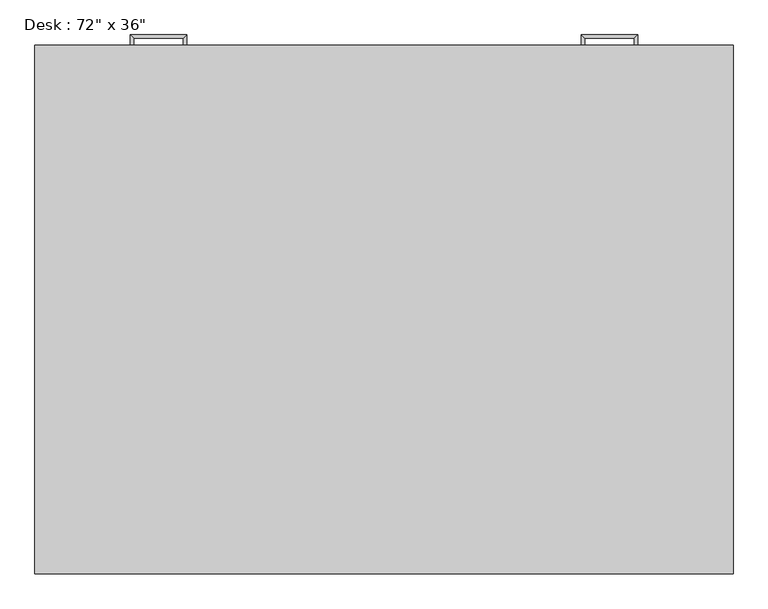
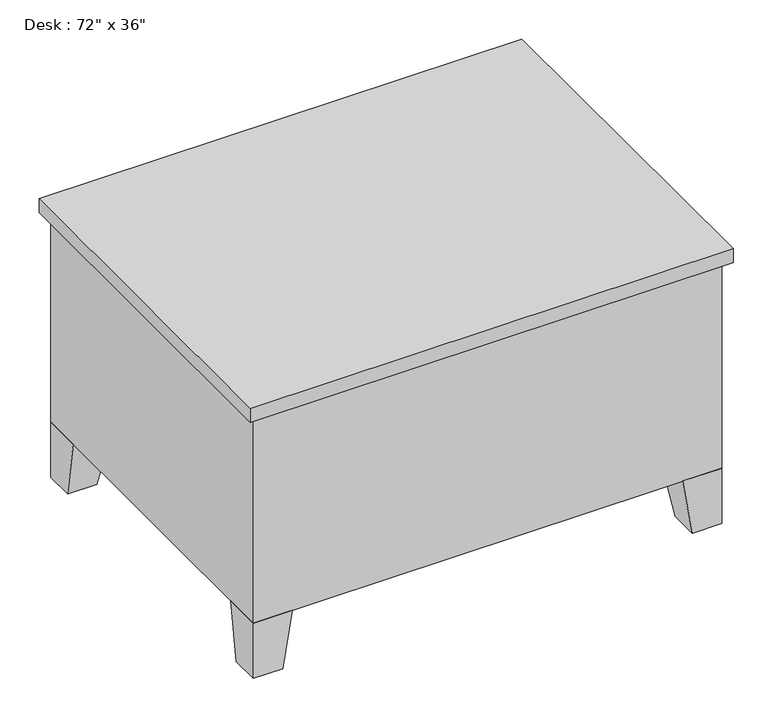
"""IFC4 building model written with IfcOpenShell, lengths in millimetres: furniture geometry."""

from ifc_helpers import new_model, si_unit, frame, origin, place, context, project, spatial, polyline, outline, extrude, faceted_brep, source, transform, mapped, element, save


def furniture_fdb83c3d(model_context):
    return source(origin(), model_context, "Body", "SolidModel", [
        extrude(outline(polyline([(1200.15, 914.4), (831.85, 914.4), (831.85, 927.1), (1200.15, 927.1), (1200.15, 914.4)])), frame((0.0, 0.0, 603.25), z_axis=(0.0, 0.0, 1.0), x_axis=(1.0, 0.0, 0.0)), (0.0, 0.0, 1.0), 101.6),
        extrude(outline(polyline([(1200.15, 914.4), (831.85, 914.4), (831.85, 927.1), (1200.15, 927.1), (1200.15, 914.4)])), frame((0.0, 0.0, 171.45), z_axis=(0.0, 0.0, 1.0), x_axis=(1.0, 0.0, 0.0)), (0.0, 0.0, 1.0), 412.75),
        extrude(outline(polyline([(387.35, 914.4), (19.05, 914.4), (19.05, 927.1), (387.35, 927.1), (387.35, 914.4)])), frame((0.0, 0.0, 603.25), z_axis=(0.0, 0.0, 1.0), x_axis=(1.0, 0.0, 0.0)), (0.0, 0.0, 1.0), 101.6),
        extrude(outline(polyline([(387.35, 914.4), (19.05, 914.4), (19.05, 927.1), (387.35, 927.1), (387.35, 914.4)])), frame((0.0, 0.0, 171.45), z_axis=(0.0, 0.0, 1.0), x_axis=(1.0, 0.0, 0.0)), (0.0, 0.0, 1.0), 171.45),
        extrude(outline(polyline([(387.35, 914.4), (19.05, 914.4), (19.05, 927.1), (387.35, 927.1), (387.35, 914.4)])), frame((0.0, 0.0, 482.6), z_axis=(0.0, 0.0, 1.0), x_axis=(1.0, 0.0, 0.0)), (0.0, 0.0, 1.0), 101.6),
        extrude(outline(polyline([(387.35, 914.4), (19.05, 914.4), (19.05, 927.1), (387.35, 927.1), (387.35, 914.4)])), frame((0.0, 0.0, 361.95), z_axis=(0.0, 0.0, 1.0), x_axis=(1.0, 0.0, 0.0)), (0.0, 0.0, 1.0), 101.6),
        faceted_brep([(1117.6, 914.4, 152.4), (1117.6, 812.8, 152.4), (1219.2, 812.8, 152.4), (1219.2, 914.4, 152.4), (1143.0, 914.4, 0.0), (1219.2, 914.4, 0.0), (1219.2, 838.2, 0.0), (1143.0, 838.2, 0.0)], [[[0, 1, 2, 3]], [[4, 5, 6, 7]], [[4, 7, 1, 0]], [[7, 6, 2, 1]], [[6, 5, 3, 2]], [[5, 4, 0, 3]]]),
        faceted_brep([(1117.6, 0.0, 152.4), (1219.2, 0.0, 152.4), (1219.2, 101.6, 152.4), (1117.6, 101.6, 152.4), (1143.0, 0.0, 0.0), (1143.0, 76.2, 0.0), (1219.2, 76.2, 0.0), (1219.2, 0.0, 0.0)], [[[0, 1, 2, 3]], [[4, 5, 6, 7]], [[4, 7, 1, 0]], [[7, 6, 2, 1]], [[6, 5, 3, 2]], [[5, 4, 0, 3]]]),
        faceted_brep([(101.6, 0.0, 152.4), (101.6, 101.6, 152.4), (0.0, 101.6, 152.4), (0.0, 0.0, 152.4), (76.2, 0.0, 0.0), (0.0, 0.0, 0.0), (0.0, 76.2, 0.0), (76.2, 76.2, 0.0)], [[[0, 1, 2, 3]], [[4, 5, 6, 7]], [[4, 7, 1, 0]], [[7, 6, 2, 1]], [[6, 5, 3, 2]], [[5, 4, 0, 3]]]),
        faceted_brep([(101.6, 914.4, 152.4), (0.0, 914.4, 152.4), (0.0, 812.8, 152.4), (101.6, 812.8, 152.4), (76.2, 914.4, 0.0), (76.2, 838.2, 0.0), (0.0, 838.2, 0.0), (0.0, 914.4, 0.0)], [[[0, 1, 2, 3]], [[4, 5, 6, 7]], [[4, 7, 1, 0]], [[7, 6, 2, 1]], [[6, 5, 3, 2]], [[5, 4, 0, 3]]]),
        extrude(outline(polyline([(1238.25, 933.45), (1238.25, -19.05), (-19.05, -19.05), (-19.05, 933.45), (1238.25, 933.45)])), frame((0.0, 0.0, 723.9), z_axis=(0.0, 0.0, 1.0), x_axis=(1.0, 0.0, 0.0)), (0.0, 0.0, 1.0), 38.1),
        extrude(outline(polyline([(406.4, 914.4), (406.4, 50.8), (812.8, 50.8), (812.8, 914.4), (1219.2, 914.4), (1219.2, 0.0), (0.0, 0.0), (0.0, 914.4), (406.4, 914.4)])), frame((0.0, 0.0, 152.4), z_axis=(0.0, 0.0, 1.0), x_axis=(1.0, 0.0, 0.0)), (0.0, 0.0, 1.0), 571.5),
        faceted_brep([(1060.45, 927.1, 546.1), (1060.45, 927.1, 533.4), (1066.8, 927.1, 533.4), (1066.8, 927.1, 546.1), (1060.45, 946.15, 546.1), (1060.45, 946.15, 533.4), (1066.8, 952.5, 533.4), (1066.8, 952.5, 546.1), (971.55, 946.15, 546.1), (971.55, 946.15, 533.4), (965.2, 952.5, 533.4), (965.2, 952.5, 546.1), (971.55, 927.1, 546.1), (965.2, 927.1, 546.1), (965.2, 927.1, 533.4), (971.55, 927.1, 533.4)], [[[0, 1, 2, 3]], [[1, 0, 4, 5]], [[2, 1, 5, 6]], [[3, 2, 6, 7]], [[0, 3, 7, 4]], [[5, 4, 8, 9]], [[6, 5, 9, 10]], [[7, 6, 10, 11]], [[4, 7, 11, 8]], [[12, 13, 14, 15]], [[9, 8, 12, 15]], [[10, 9, 15, 14]], [[11, 10, 14, 13]], [[8, 11, 13, 12]]]),
        faceted_brep([(1060.45, 927.1, 666.75), (1060.45, 927.1, 654.05), (1066.8, 927.1, 654.05), (1066.8, 927.1, 666.75), (1060.45, 946.15, 666.75), (1060.45, 946.15, 654.05), (1066.8, 952.5, 654.05), (1066.8, 952.5, 666.75), (971.55, 946.15, 666.75), (971.55, 946.15, 654.05), (965.2, 952.5, 654.05), (965.2, 952.5, 666.75), (971.55, 927.1, 666.75), (965.2, 927.1, 666.75), (965.2, 927.1, 654.05), (971.55, 927.1, 654.05)], [[[0, 1, 2, 3]], [[1, 0, 4, 5]], [[2, 1, 5, 6]], [[3, 2, 6, 7]], [[0, 3, 7, 4]], [[5, 4, 8, 9]], [[6, 5, 9, 10]], [[7, 6, 10, 11]], [[4, 7, 11, 8]], [[12, 13, 14, 15]], [[9, 8, 12, 15]], [[10, 9, 15, 14]], [[11, 10, 14, 13]], [[8, 11, 13, 12]]]),
        faceted_brep([(158.75, 927.1, 304.8), (152.4, 927.1, 304.8), (152.4, 927.1, 292.1), (158.75, 927.1, 292.1), (158.75, 946.15, 304.8), (152.4, 952.5, 304.8), (152.4, 952.5, 292.1), (158.75, 946.15, 292.1), (247.65, 946.15, 304.8), (254.0, 952.5, 304.8), (254.0, 952.5, 292.1), (247.65, 946.15, 292.1), (247.65, 927.1, 304.8), (247.65, 927.1, 292.1), (254.0, 927.1, 292.1), (254.0, 927.1, 304.8)], [[[0, 1, 2, 3]], [[1, 0, 4, 5]], [[2, 1, 5, 6]], [[3, 2, 6, 7]], [[0, 3, 7, 4]], [[5, 4, 8, 9]], [[6, 5, 9, 10]], [[7, 6, 10, 11]], [[4, 7, 11, 8]], [[12, 13, 14, 15]], [[9, 8, 12, 15]], [[10, 9, 15, 14]], [[11, 10, 14, 13]], [[8, 11, 13, 12]]]),
        faceted_brep([(158.75, 927.1, 425.45), (152.4, 927.1, 425.45), (152.4, 927.1, 412.75), (158.75, 927.1, 412.75), (158.75, 946.15, 425.45), (152.4, 952.5, 425.45), (152.4, 952.5, 412.75), (158.75, 946.15, 412.75), (247.65, 946.15, 425.45), (254.0, 952.5, 425.45), (254.0, 952.5, 412.75), (247.65, 946.15, 412.75), (247.65, 927.1, 425.45), (247.65, 927.1, 412.75), (254.0, 927.1, 412.75), (254.0, 927.1, 425.45)], [[[0, 1, 2, 3]], [[1, 0, 4, 5]], [[2, 1, 5, 6]], [[3, 2, 6, 7]], [[0, 3, 7, 4]], [[5, 4, 8, 9]], [[6, 5, 9, 10]], [[7, 6, 10, 11]], [[4, 7, 11, 8]], [[12, 13, 14, 15]], [[9, 8, 12, 15]], [[10, 9, 15, 14]], [[11, 10, 14, 13]], [[8, 11, 13, 12]]]),
        faceted_brep([(158.75, 927.1, 546.1), (152.4, 927.1, 546.1), (152.4, 927.1, 533.4), (158.75, 927.1, 533.4), (158.75, 946.15, 546.1), (152.4, 952.5, 546.1), (152.4, 952.5, 533.4), (158.75, 946.15, 533.4), (247.65, 946.15, 546.1), (254.0, 952.5, 546.1), (254.0, 952.5, 533.4), (247.65, 946.15, 533.4), (247.65, 927.1, 546.1), (247.65, 927.1, 533.4), (254.0, 927.1, 533.4), (254.0, 927.1, 546.1)], [[[0, 1, 2, 3]], [[1, 0, 4, 5]], [[2, 1, 5, 6]], [[3, 2, 6, 7]], [[0, 3, 7, 4]], [[5, 4, 8, 9]], [[6, 5, 9, 10]], [[7, 6, 10, 11]], [[4, 7, 11, 8]], [[12, 13, 14, 15]], [[9, 8, 12, 15]], [[10, 9, 15, 14]], [[11, 10, 14, 13]], [[8, 11, 13, 12]]]),
        faceted_brep([(158.75, 927.1, 666.75), (152.4, 927.1, 666.75), (152.4, 927.1, 654.05), (158.75, 927.1, 654.05), (158.75, 946.15, 666.75), (152.4, 952.5, 666.75), (152.4, 952.5, 654.05), (158.75, 946.15, 654.05), (247.65, 946.15, 666.75), (254.0, 952.5, 666.75), (254.0, 952.5, 654.05), (247.65, 946.15, 654.05), (247.65, 927.1, 666.75), (247.65, 927.1, 654.05), (254.0, 927.1, 654.05), (254.0, 927.1, 666.75)], [[[0, 1, 2, 3]], [[1, 0, 4, 5]], [[2, 1, 5, 6]], [[3, 2, 6, 7]], [[0, 3, 7, 4]], [[5, 4, 8, 9]], [[6, 5, 9, 10]], [[7, 6, 10, 11]], [[4, 7, 11, 8]], [[12, 13, 14, 15]], [[9, 8, 12, 15]], [[10, 9, 15, 14]], [[11, 10, 14, 13]], [[8, 11, 13, 12]]]),
    ])


if __name__ == "__main__":
    model = new_model("IFC4")
    model_context = context("Model", 3, world=origin())
    ifc_project = project(units=[si_unit("LENGTHUNIT", "METRE", prefix="MILLI")], contexts=[model_context])
    site = spatial("IfcSite", under=ifc_project)
    building = spatial("IfcBuilding", under=site)
    placement = place(None, origin())
    furniture_shape = furniture_fdb83c3d(model_context)
    element("IfcFurniture", 1, ObjectType="Desk : 72\" x 36\"", at=placement, inside=building, context=model_context, shape_type="MappedRepresentation", body=[
        mapped(furniture_shape, transform((0.0, 0.0, 0.0), x_axis=(1.0, 0.0, 0.0), y_axis=(0.0, 1.0, 0.0), z_axis=(0.0, 0.0, 1.0))),
    ])
    save(model, "model.ifc")

# Revit data of these elements
# Type "Desk : 72\" x 36\""
#   Assembly Code = "E2020200"
#   Depth = 3' - 0"
#   Height = 2' - 6"
#   Leg Height = 0' - 6"
#   Width = 4' - 0"
#   Body Material = Laminate, Ivory, Matte
#   Handle/Leg Material = Steel, Chrome Plated
#   Top Material = Cherry
#   Default Elevation = 0
# Element 1 (IfcFurniture, "Desk : 72\" x 36\"")
#   Materials on its faces: "Steel, Chrome Plated", "Laminate, Ivory, Matte", "Cherry"
# Materials
#   "Laminate, Ivory, Matte": class "Plastic", colour RGB 247 247 239, transparency 0, Description = "Plastic Laminate - Ivory, Matte", Cost = 0
#   "Steel, Chrome Plated": class "Metal", colour RGB 17 17 17, transparency 0, Description = "Chromiuim plated steel", Cost = 0
#   "Cherry": class "Wood", colour RGB 226 177 128, transparency 0, Description = "Prunus Serotina", Cost = 0
